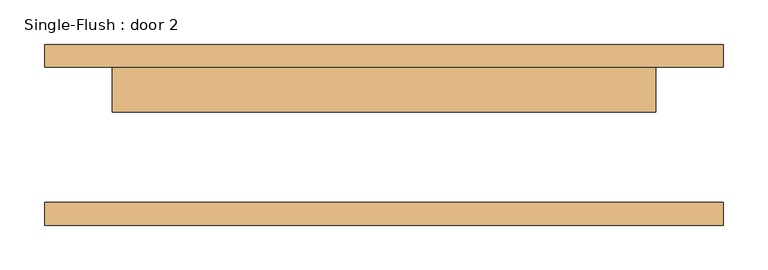
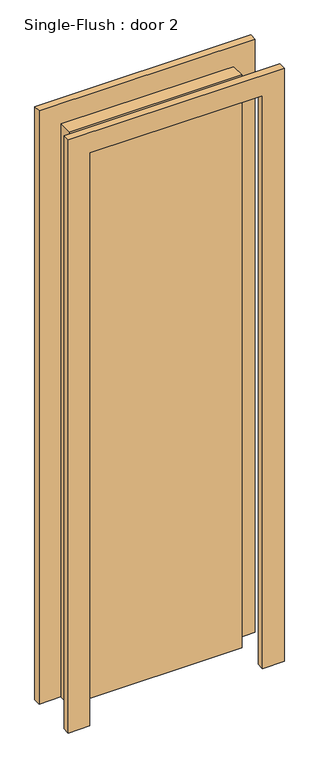
"""IFC4 building model written with IfcOpenShell, lengths in millimetres: door geometry, Single-Flush : door 2."""

from ifc_helpers import new_model, si_unit, frame, origin, origin_with_axes, place, context, project, spatial, polyline, outline, extrude, source, transform, mapped, element, save


def single_flush_door_2_9ea4ff49(model_context):
    return source(origin(), model_context, "Body", "SweptSolid", [
        extrude(outline(polyline([(2209.8, -381.0), (0.0, -381.0), (0.0, -304.8), (2133.6, -304.8), (2133.6, 304.8), (0.0, 304.8), (0.0, 381.0), (2209.8, 381.0), (2209.8, -381.0)])), frame((0.0, 76.2, 0.0), z_axis=(0.0, 1.0, 0.0), x_axis=(0.0, 0.0, 1.0)), (0.0, 0.0, 1.0), 25.4),
        extrude(outline(polyline([(2209.8, 381.0), (2209.8, -381.0), (0.0, -381.0), (0.0, -304.8), (2133.6, -304.8), (2133.6, 304.8), (0.0, 304.8), (0.0, 381.0), (2209.8, 381.0)])), frame((0.0, -101.6, 0.0), z_axis=(0.0, 1.0, 0.0), x_axis=(0.0, 0.0, 1.0)), (0.0, 0.0, 1.0), 25.4),
        extrude(outline(polyline([(304.8, 25.4), (-304.8, 25.4), (-304.8, 76.2), (304.8, 76.2), (304.8, 25.4)])), origin_with_axes(), (0.0, 0.0, 1.0), 2133.6),
    ])


if __name__ == "__main__":
    model = new_model("IFC4")
    model_context = context("Model", 3, world=origin())
    ifc_project = project(units=[si_unit("LENGTHUNIT", "METRE", prefix="MILLI")], contexts=[model_context])
    site = spatial("IfcSite", under=ifc_project)
    building = spatial("IfcBuilding", under=site)
    placement = place(None, origin())
    single_flush_door_2_shape = single_flush_door_2_9ea4ff49(model_context)
    element("IfcDoor", 1, ObjectType="Single-Flush : door 2", at=placement, inside=building, context=model_context, shape_type="MappedRepresentation", body=[
        mapped(single_flush_door_2_shape, transform((0.0, 0.0, 0.0), x_axis=(1.0, 0.0, 0.0), y_axis=(0.0, 1.0, 0.0), z_axis=(0.0, 0.0, 1.0))),
    ])
    save(model, "model.ifc")

# Revit data of these elements
# Type "Single-Flush : door 2"
#   Type Mark = "8"
#   Construction Type Id = "MDOOR"
#   Assembly Code = "C1020"
#   Analytic Construction = "Metal"
#   Thickness = 0' - 2"
#   Heat Transfer Coefficient (U) = 0.651978 BTU/(h·ft²·°F)
#   Height = 7' - 0"
#   Trim Projection Ext = 0' - 1"
#   Trim Projection Int = 0' - 1"
#   Trim Width = 0' - 3"
#   Width = 2' - 0"
#   Define Thermal Properties by = 1
#   Door Material = Door - Panel
#   Frame Material = Door - Frame
#   Visual Light Transmittance = 0
#   Solar Heat Gain Coefficient = 0
#   Function = (empty or 0)
#   Wall Closure = (empty or 0)
# Element 1 (IfcDoor, "Single-Flush : door 2")
#   Materials on its faces: "Door - Frame", "Door - Panel"
# Materials
#   "Door - Panel": class "Wood", colour RGB 210 159 95, transparency 0
#   "Door - Frame": colour RGB 118 70 51, transparency 0
